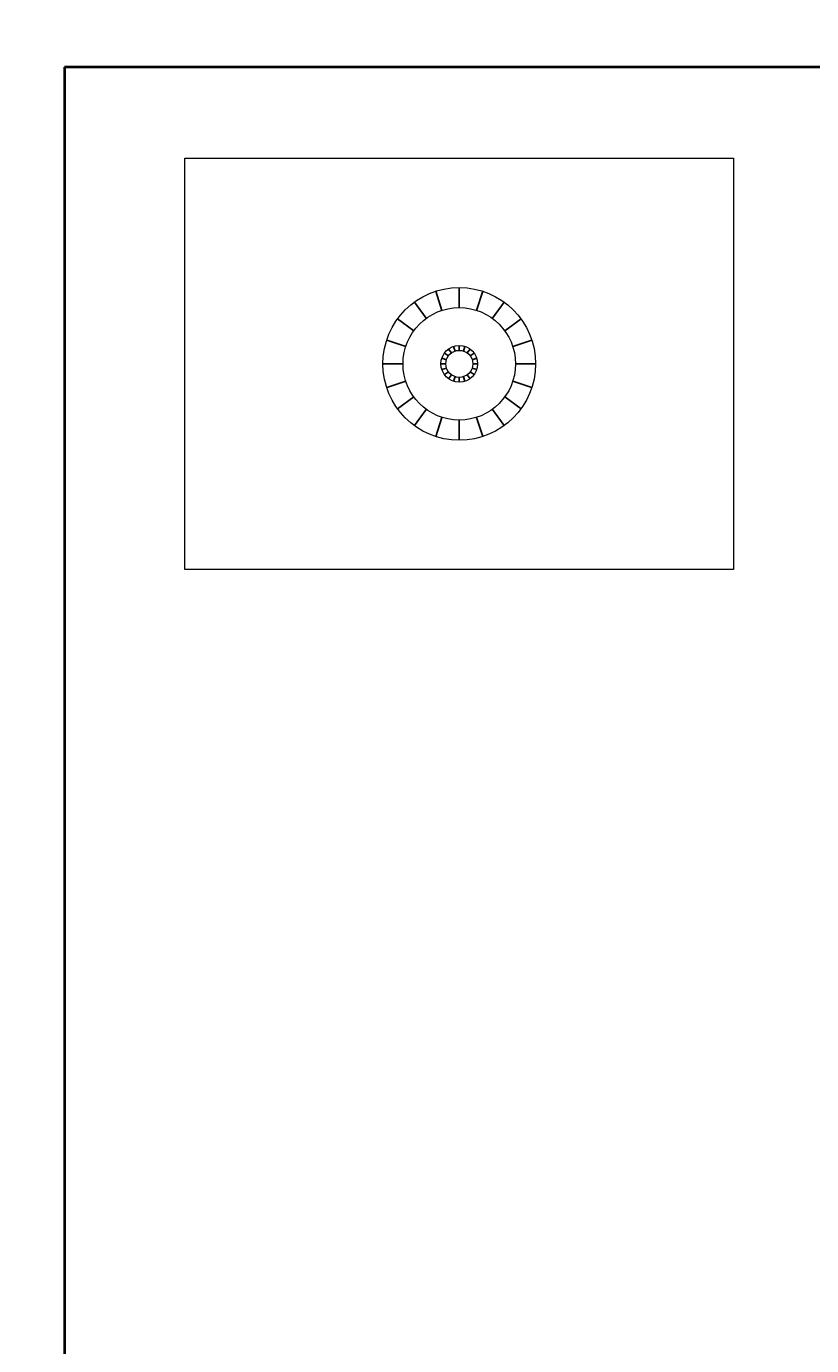
# Model space of a CAD drawing. Units: inches. Extents: x -46 to 1145, y -527 to 760.
# Tile 37 of 57: x 20 to 53, y 597 to 652. Entities that reach past the tile are written whole.
import ezdxf

# ---------------------------------------------------------------- set-up
doc = ezdxf.new("R2010")
doc.units = ezdxf.units.IN
doc.header["$MEASUREMENT"] = 0
for name, color, linetype, lineweight in [('A-ANNO-DIMS', 2, 'Continuous', 18), ('A-FURN', 2, 'Continuous', 13), ('WALLS', 4, 'Continuous', 40)]:
    doc.layers.add(name, color=color, linetype=linetype, lineweight=lineweight)
doc.layers.add('FURNTIURE', color=2, linetype='Continuous')
doc.styles.get("Standard").update_dxf_attribs({"font": 'arial.ttf'})
doc.dimstyles.get("Standard").update_dxf_attribs({"dimtxt": 0.18, "dimasz": 0.18, "dimexe": 0.18, "dimexo": 0.0625, "dimgap": 0.09, "dimtad": 0, "dimtih": 1, "dimtoh": 1, "dimdec": 0, "dimzin": 0, "dimdsep": 46, "dimlunit": 3, "dimtxsty": 'Standard', "dimcen": 0.09, "dimadec": 0, "dimazin": 0, "dimtfac": 1, "dimtdec": 0, "dimtofl": 0, "dimtmove": 0, "dimatfit": 3, "dimfxl": 1, "dimtolj": 1, "dimtzin": 0, "dimarcsym": 0})

# ---------------------------------------------------------------- blocks, each defined once
blk = doc.blocks.new('*U89')
at = {"layer": 'FURNTIURE'}
blk.add_line((0, 0.422), (0, -0.422), dxfattribs=at)
blk = doc.blocks.new('*U90')
at = {"layer": 'FURNTIURE', "transparency": 16777216}
for p, rotation in [((590.891, 507.397), 17.99999999999997), ((592.613, 507.397), 341.9999999999999), ((590.114, 507.002), 36), ((593.39, 507.002), 324), ((589.498, 506.385), 54), ((594.007, 506.385), 306), ((589.102, 505.608), 72), ((594.402, 505.608), 288), ((588.965, 504.747), 90), ((594.539, 504.747), 270), ((589.102, 503.886), 108), ((594.402, 503.886), 252), ((589.498, 503.109), 126), ((594.007, 503.109), 234), ((590.114, 502.493), 144), ((593.39, 502.493), 216), ((590.891, 502.097), 162), ((591.752, 501.961), 180), ((592.613, 502.097), 197.9999999999999)]:
    blk.add_blockref('*U89', p, dxfattribs=dict(at, rotation=rotation))
blk.add_blockref('*U89', (591.752, 507.534), dxfattribs=at)
blk = doc.blocks.new('*U87')
at = {"layer": 'FURNTIURE'}
blk.add_line((0, 0.101), (0, -0.101), dxfattribs=at)
blk = doc.blocks.new('*U88')
at = {"layer": 'FURNTIURE', "transparency": 16777216}
for p, rotation in [((141.362, 121.431), 54), ((141.51, 121.579), 35.99999999999999), ((141.696, 121.674), 17.99999999999998), ((142.109, 121.674), 342), ((142.295, 121.579), 324), ((142.443, 121.431), 306), ((141.234, 121.039), 90), ((141.267, 121.245), 72), ((141.267, 120.832), 108), ((142.538, 121.245), 288), ((142.538, 120.832), 252), ((142.571, 121.039), 270), ((141.362, 120.646), 126), ((141.51, 120.498), 144), ((141.696, 120.403), 162), ((141.902, 120.37), 180), ((142.109, 120.403), 198), ((142.295, 120.498), 216), ((142.443, 120.646), 234)]:
    blk.add_blockref('*U87', p, dxfattribs=dict(at, rotation=rotation))
blk.add_blockref('*U87', (141.902, 121.707), dxfattribs=at)
blk = doc.blocks.new('NIGHTSTAND')
blk.add_lwpolyline([(23.061, 0), (0, 0), (0, 17.285), (23.061, 17.285)], close=True)
for radius in [3.209, 2.364, 0.77, 0.567]:
    blk.add_circle((11.53, 8.643), radius)
for name, p in [('*U90', (-580.222, -496.105)), ('*U88', (-130.372, -112.396))]:
    blk.add_blockref(name, p)
blk = doc.blocks.new('*D685')
at = {"layer": 'A-ANNO-DIMS', "color": 0, "lineweight": -2, "transparency": 16777216}
for p, q in [((183.501, 700.889), (-46.216, 700.889)), ((-46.036, 700.709), (-46.036, 116.385)), ((-46.036, -468.302), (-46.036, 116.021)), ((12.501, -468.482), (-46.216, -468.482))]:
    blk.add_line(p, q, dxfattribs=at)
at = {"layer": 'A-ANNO-DIMS', "color": 0, "transparency": 16777216}
for points in [[(-46.066, 700.709), (-46.006, 700.709), (-46.036, 700.889)], [(-46.066, -468.302), (-46.006, -468.302), (-46.036, -468.482)]]:
    blk.add_solid(points, dxfattribs=at)
at = {"layer": 'Defpoints', "color": 0, "transparency": 16777216}
for p in [(-46.036, 700.889), (183.564, 700.889), (12.564, -468.482)]:
    blk.add_point(p, dxfattribs=at)
at = {"layer": 'A-ANNO-DIMS', "color": 0, "transparency": 16777216, "insert": (-46.036, 116.203), "char_height": 0.18, "attachment_point": 5}
blk.add_mtext('\\A1;1169.4', dxfattribs=at)

msp = doc.modelspace()

# ---------------------------------------------------------------- linework, layer by layer
at = {"layer": 'WALLS'}
for p, q in [((21.5637, 650.5176), (21.5637, 506.5176)), ((183.5637, 650.5176), (21.5637, 650.5176))]:
    msp.add_line(p, q, dxfattribs=at)

# ---------------------------------------------------------------- block references
at = {"layer": 'A-FURN'}
msp.add_blockref('NIGHTSTAND', (26.626, 629.415), dxfattribs=at)

# ---------------------------------------------------------------- dimensions: what is measured, and where the dimension line sits
at = {"layer": 'A-ANNO-DIMS'}
dim = msp.add_linear_dim(base=(-46.0363, 700.8886), p1=(12.5637, -468.4824), p2=(183.5637, 700.8886), angle=90, dimstyle='Standard', override={"dimdec": 1, "dimlfac": 1, "dimrnd": 0, "dimzin": 0, "dimdsep": 46, "dimlunit": 2}, dxfattribs=at)
dim.commit()
dim.dimension.update_dxf_attribs({"geometry": '*D685', "text_midpoint": (-46.0363, 116.2031)})

doc.saveas('drawing.dxf')
